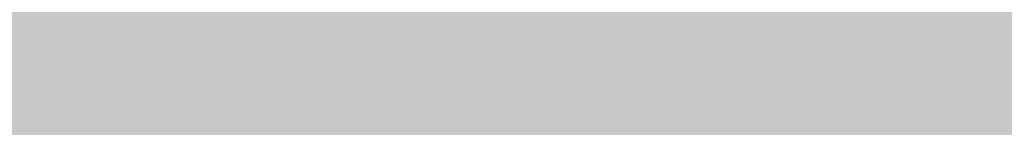
# Model space of a CAD drawing. Units: millimetres. Extents: x -22994 to 29398, y -19990 to 20176.
# Tile 71 of 135: x 226.355 to 227.437, y 83.328 to 83.446. Entities that reach past the tile are written whole.
import ezdxf
from ezdxf import colors
from ezdxf.entities.mleader import LeaderData, LeaderLine
from ezdxf.math import Vec2, Vec3

# ---------------------------------------------------------------- set-up
doc = ezdxf.new("R2010")
doc.units = ezdxf.units.MM
doc.header["$MEASUREMENT"] = 0
doc.layers.add('M-ANNO-TEXT', color=7, linetype='Continuous', lineweight=25)
doc.layers.add('M-DIMS', color=2, linetype='Continuous', lineweight=18)
doc.styles.get("Standard").update_dxf_attribs({"font": 'arial.ttf'})
doc.dimstyles.get("Standard").update_dxf_attribs({"dimtxt": 0.18, "dimasz": 10000, "dimexe": 0.18, "dimexo": 0.0625, "dimgap": 0.09, "dimtad": 0, "dimtih": 1, "dimtoh": 1, "dimdec": 0, "dimzin": 0, "dimdsep": 46, "dimtxsty": 'Standard', "dimcen": 0.09, "dimadec": 0, "dimazin": 0, "dimtfac": 1, "dimtdec": 0, "dimtofl": 0, "dimtmove": 0, "dimatfit": 3, "dimfxl": 1, "dimtolj": 1, "dimtzin": 0, "dimlwd": 30, "dimarcsym": 0})

# ---------------------------------------------------------------- blocks, each defined once
blk = doc.blocks.new('*D2')
at = {"layer": 'Defpoints', "color": 0, "transparency": 16777216}
for p in [(6.6773, 10.2713), (290.852, 10.2713), (290.852, -5.0787)]:
    blk.add_point(p, dxfattribs=at)
at = {"layer": 'M-DIMS', "color": 0, "lineweight": -2, "transparency": 16777216}
for p, q in [((6.6773, 10.2088), (6.6773, -5.2587)), ((290.852, 10.2088), (290.852, -5.2587))]:
    blk.add_line(p, q, dxfattribs=at)
at = {"layer": 'M-DIMS', "color": 0, "lineweight": 30, "transparency": 16777216}
for p, q in [((-9993.3227, -5.0787), (-19993.3227, -5.0787)), ((10290.852, -5.0787), (20290.852, -5.0787))]:
    blk.add_line(p, q, dxfattribs=at)
at = {"layer": 'M-DIMS', "color": 0, "transparency": 16777216}
for points in [[(-9993.3227, 1661.5879), (-9993.3227, -1671.7454), (6.6773, -5.0787)], [(10290.852, 1661.5879), (10290.852, -1671.7454), (290.852, -5.0787)]]:
    blk.add_solid(points, dxfattribs=at)
at = {"layer": 'M-DIMS', "color": 0, "transparency": 16777216, "insert": (148.7647, -5.0787), "char_height": 0.18, "attachment_point": 5}
blk.add_mtext('\\A1;284.2', dxfattribs=at)
blk = doc.blocks.new('*D3')
at = {"layer": 'Defpoints', "color": 0, "transparency": 16777216}
for p in [(110.2647, 204.1654), (110.2647, 176.3662), (95.8327, 127.967)]:
    blk.add_point(p, dxfattribs=at)
at = {"layer": 'M-DIMS', "color": 0, "lineweight": -2, "transparency": 16777216}
for p, q in [((95.8327, 128.0295), (95.8327, 204.3454)), ((110.2647, 176.4287), (110.2647, 204.3454))]:
    blk.add_line(p, q, dxfattribs=at)
at = {"layer": 'M-DIMS', "color": 0, "lineweight": 30, "transparency": 16777216}
for p, q in [((-9904.1673, 204.1654), (-19904.1673, 204.1654)), ((10110.2647, 204.1654), (20110.2647, 204.1654))]:
    blk.add_line(p, q, dxfattribs=at)
at = {"layer": 'M-DIMS', "color": 0, "transparency": 16777216}
for points in [[(-9904.1673, 1870.8321), (-9904.1673, -1462.5013), (95.8327, 204.1654)], [(10110.2647, 1870.8321), (10110.2647, -1462.5013), (110.2647, 204.1654)]]:
    blk.add_solid(points, dxfattribs=at)
at = {"layer": 'M-DIMS', "color": 0, "transparency": 16777216, "insert": (103.0487, 204.1654), "char_height": 0.18, "attachment_point": 5}
blk.add_mtext('\\A1;14.432', dxfattribs=at)
blk = doc.blocks.new('*D4')
at = {"layer": 'Defpoints', "color": 0, "transparency": 16777216}
for p in [(116.2647, 204.1654), (110.2647, 176.3662), (116.2647, 176.3662)]:
    blk.add_point(p, dxfattribs=at)
at = {"layer": 'M-DIMS', "color": 0, "lineweight": -2, "transparency": 16777216}
for p, q in [((110.2647, 176.4287), (110.2647, 204.3454)), ((116.2647, 176.4287), (116.2647, 204.3454))]:
    blk.add_line(p, q, dxfattribs=at)
at = {"layer": 'M-DIMS', "color": 0, "lineweight": 30, "transparency": 16777216}
for p, q in [((-9889.7353, 204.1654), (-19889.7353, 204.1654)), ((10116.2647, 204.1654), (20116.2647, 204.1654))]:
    blk.add_line(p, q, dxfattribs=at)
at = {"layer": 'M-DIMS', "color": 0, "transparency": 16777216}
for points in [[(-9889.7353, 1870.8321), (-9889.7353, -1462.5013), (110.2647, 204.1654)], [(10116.2647, 1870.8321), (10116.2647, -1462.5013), (116.2647, 204.1654)]]:
    blk.add_solid(points, dxfattribs=at)
at = {"layer": 'M-DIMS', "color": 0, "transparency": 16777216, "insert": (113.2647, 204.1654), "char_height": 0.18, "attachment_point": 5}
blk.add_mtext('\\A1;6', dxfattribs=at)
blk = doc.blocks.new('*D5')
at = {"layer": 'Defpoints', "color": 0, "transparency": 16777216}
for p in [(181.2647, 204.1654), (116.2647, 176.3662), (181.2647, 176.3662)]:
    blk.add_point(p, dxfattribs=at)
at = {"layer": 'M-DIMS', "color": 0, "lineweight": -2, "transparency": 16777216}
for p, q in [((116.2647, 176.4287), (116.2647, 204.3454)), ((181.2647, 176.4287), (181.2647, 204.3454))]:
    blk.add_line(p, q, dxfattribs=at)
at = {"layer": 'M-DIMS', "color": 0, "lineweight": 30, "transparency": 16777216}
for p, q in [((-9883.7353, 204.1654), (-19883.7353, 204.1654)), ((10181.2647, 204.1654), (20181.2647, 204.1654))]:
    blk.add_line(p, q, dxfattribs=at)
at = {"layer": 'M-DIMS', "color": 0, "transparency": 16777216}
for points in [[(-9883.7353, 1870.8321), (-9883.7353, -1462.5013), (116.2647, 204.1654)], [(10181.2647, 1870.8321), (10181.2647, -1462.5013), (181.2647, 204.1654)]]:
    blk.add_solid(points, dxfattribs=at)
at = {"layer": 'M-DIMS', "color": 0, "transparency": 16777216, "insert": (148.7647, 204.1654), "char_height": 0.18, "attachment_point": 5}
blk.add_mtext('\\A1;65', dxfattribs=at)
blk = doc.blocks.new('*D6')
at = {"layer": 'Defpoints', "color": 0, "transparency": 16777216}
for p in [(187.2647, 204.1654), (181.2647, 176.3662), (187.2647, 176.3662)]:
    blk.add_point(p, dxfattribs=at)
at = {"layer": 'M-DIMS', "color": 0, "lineweight": -2, "transparency": 16777216}
for p, q in [((181.2647, 176.4287), (181.2647, 204.3454)), ((187.2647, 176.4287), (187.2647, 204.3454))]:
    blk.add_line(p, q, dxfattribs=at)
at = {"layer": 'M-DIMS', "color": 0, "lineweight": 30, "transparency": 16777216}
for p, q in [((-9818.7353, 204.1654), (-19818.7353, 204.1654)), ((10187.2647, 204.1654), (20187.2647, 204.1654))]:
    blk.add_line(p, q, dxfattribs=at)
at = {"layer": 'M-DIMS', "color": 0, "transparency": 16777216}
for points in [[(-9818.7353, 1870.8321), (-9818.7353, -1462.5013), (181.2647, 204.1654)], [(10187.2647, 1870.8321), (10187.2647, -1462.5013), (187.2647, 204.1654)]]:
    blk.add_solid(points, dxfattribs=at)
at = {"layer": 'M-DIMS', "color": 0, "transparency": 16777216, "insert": (184.2647, 204.1654), "char_height": 0.18, "attachment_point": 5}
blk.add_mtext('\\A1;6', dxfattribs=at)
blk = doc.blocks.new('*D7')
at = {"layer": 'Defpoints', "color": 0, "transparency": 16777216}
for p in [(201.6967, 204.1654), (187.2647, 176.3662), (201.6967, 127.967)]:
    blk.add_point(p, dxfattribs=at)
at = {"layer": 'M-DIMS', "color": 0, "lineweight": -2, "transparency": 16777216}
for p, q in [((187.2647, 176.4287), (187.2647, 204.3454)), ((201.6967, 128.0295), (201.6967, 204.3454))]:
    blk.add_line(p, q, dxfattribs=at)
at = {"layer": 'M-DIMS', "color": 0, "lineweight": 30, "transparency": 16777216}
for p, q in [((-9812.7353, 204.1654), (-19812.7353, 204.1654)), ((10201.6967, 204.1654), (20201.6967, 204.1654))]:
    blk.add_line(p, q, dxfattribs=at)
at = {"layer": 'M-DIMS', "color": 0, "transparency": 16777216}
for points in [[(-9812.7353, 1870.8321), (-9812.7353, -1462.5013), (187.2647, 204.1654)], [(10201.6967, 1870.8321), (10201.6967, -1462.5013), (201.6967, 204.1654)]]:
    blk.add_solid(points, dxfattribs=at)
at = {"layer": 'M-DIMS', "color": 0, "transparency": 16777216, "insert": (194.4807, 204.1654), "char_height": 0.18, "attachment_point": 5}
blk.add_mtext('\\A1;14.432', dxfattribs=at)
blk = doc.blocks.new('*D8')
at = {"layer": 'Defpoints', "color": 0, "transparency": 16777216}
for p in [(227.6485, 204.1654), (227.6485, 146.7296), (201.6967, 127.967)]:
    blk.add_point(p, dxfattribs=at)
at = {"layer": 'M-DIMS', "color": 0, "lineweight": -2, "transparency": 16777216}
for p, q in [((201.6967, 128.0295), (201.6967, 204.3454)), ((227.6485, 146.7921), (227.6485, 204.3454))]:
    blk.add_line(p, q, dxfattribs=at)
at = {"layer": 'M-DIMS', "color": 0, "lineweight": 30, "transparency": 16777216}
for p, q in [((-9798.3033, 204.1654), (-19798.3033, 204.1654)), ((10227.6485, 204.1654), (20227.6485, 204.1654))]:
    blk.add_line(p, q, dxfattribs=at)
at = {"layer": 'M-DIMS', "color": 0, "transparency": 16777216}
for points in [[(-9798.3033, 1870.8321), (-9798.3033, -1462.5013), (201.6967, 204.1654)], [(10227.6485, 1870.8321), (10227.6485, -1462.5013), (227.6485, 204.1654)]]:
    blk.add_solid(points, dxfattribs=at)
at = {"layer": 'M-DIMS', "color": 0, "transparency": 16777216, "insert": (214.6726, 204.1654), "char_height": 0.18, "attachment_point": 5}
blk.add_mtext('\\A1;25.95', dxfattribs=at)
blk = doc.blocks.new('*D9')
at = {"layer": 'Defpoints', "color": 0, "transparency": 16777216}
for p in [(187.2647, 176.3662), (306.202, 176.3662), (290.852, 10.2713)]:
    blk.add_point(p, dxfattribs=at)
at = {"layer": 'M-DIMS', "color": 0, "lineweight": 30, "transparency": 16777216}
for p, q in [((306.202, 10176.3662), (306.202, 20176.3662)), ((306.202, -9989.7287), (306.202, -19989.7287))]:
    blk.add_line(p, q, dxfattribs=at)
at = {"layer": 'M-DIMS', "color": 0, "lineweight": -2, "transparency": 16777216}
for p, q in [((187.3272, 176.3662), (306.382, 176.3662)), ((290.9145, 10.2713), (306.382, 10.2713))]:
    blk.add_line(p, q, dxfattribs=at)
at = {"layer": 'M-DIMS', "color": 0, "transparency": 16777216}
for points in [[(-1360.4646, 10176.3662), (1972.8687, 10176.3662), (306.202, 176.3662)], [(-1360.4646, -9989.7287), (1972.8687, -9989.7287), (306.202, 10.2713)]]:
    blk.add_solid(points, dxfattribs=at)
at = {"layer": 'M-DIMS', "color": 0, "transparency": 16777216, "insert": (306.202, 93.3187), "char_height": 0.18, "attachment_point": 5}
blk.add_mtext('\\A1;166.1', dxfattribs=at)
blk = doc.blocks.new('*D10')
at = {"layer": 'Defpoints', "color": 0, "transparency": 16777216}
for p in [(125.6498, 136.0713), (133.3459, 136.0713), (133.3459, -5.0787)]:
    blk.add_point(p, dxfattribs=at)
at = {"layer": 'M-DIMS', "color": 0, "lineweight": -2, "transparency": 16777216}
for p, q in [((125.6498, 136.0088), (125.6498, -5.2587)), ((133.3459, 136.0088), (133.3459, -5.2587))]:
    blk.add_line(p, q, dxfattribs=at)
at = {"layer": 'M-DIMS', "color": 0, "lineweight": 30, "transparency": 16777216}
for p, q in [((-9874.3502, -5.0787), (-19874.3502, -5.0787)), ((10133.3459, -5.0787), (20133.3459, -5.0787))]:
    blk.add_line(p, q, dxfattribs=at)
at = {"layer": 'M-DIMS', "color": 0, "transparency": 16777216}
for points in [[(-9874.3502, 1661.5879), (-9874.3502, -1671.7454), (125.6498, -5.0787)], [(10133.3459, 1661.5879), (10133.3459, -1671.7454), (133.3459, -5.0787)]]:
    blk.add_solid(points, dxfattribs=at)
at = {"layer": 'M-DIMS', "color": 0, "transparency": 16777216, "insert": (129.4978, -5.0787), "char_height": 0.18, "attachment_point": 5}
blk.add_mtext('\\A1;7.696', dxfattribs=at)
blk = doc.blocks.new('*D11')
at = {"layer": 'Defpoints', "color": 0, "transparency": 16777216}
for p in [(133.3459, 136.0713), (135.6498, 136.0713), (135.6498, -5.0787)]:
    blk.add_point(p, dxfattribs=at)
at = {"layer": 'M-DIMS', "color": 0, "lineweight": -2, "transparency": 16777216}
for p, q in [((133.3459, 136.0088), (133.3459, -5.2587)), ((135.6498, 136.0088), (135.6498, -5.2587))]:
    blk.add_line(p, q, dxfattribs=at)
at = {"layer": 'M-DIMS', "color": 0, "lineweight": 30, "transparency": 16777216}
for p, q in [((-9866.6541, -5.0787), (-19866.6541, -5.0787)), ((10135.6498, -5.0787), (20135.6498, -5.0787))]:
    blk.add_line(p, q, dxfattribs=at)
at = {"layer": 'M-DIMS', "color": 0, "transparency": 16777216}
for points in [[(-9866.6541, 1661.5879), (-9866.6541, -1671.7454), (133.3459, -5.0787)], [(10135.6498, 1661.5879), (10135.6498, -1671.7454), (135.6498, -5.0787)]]:
    blk.add_solid(points, dxfattribs=at)
at = {"layer": 'M-DIMS', "color": 0, "transparency": 16777216, "insert": (134.4978, -5.0787), "char_height": 0.18, "attachment_point": 5}
blk.add_mtext('\\A1;2.304', dxfattribs=at)
blk = doc.blocks.new('*D12')
at = {"layer": 'Defpoints', "color": 0, "transparency": 16777216}
for p in [(135.6498, 136.0713), (145.6498, 136.0713), (145.6498, -5.0787)]:
    blk.add_point(p, dxfattribs=at)
at = {"layer": 'M-DIMS', "color": 0, "lineweight": -2, "transparency": 16777216}
for p, q in [((135.6498, 136.0088), (135.6498, -5.2587)), ((145.6498, 136.0088), (145.6498, -5.2587))]:
    blk.add_line(p, q, dxfattribs=at)
at = {"layer": 'M-DIMS', "color": 0, "lineweight": 30, "transparency": 16777216}
for p, q in [((-9864.3502, -5.0787), (-19864.3502, -5.0787)), ((10145.6498, -5.0787), (20145.6498, -5.0787))]:
    blk.add_line(p, q, dxfattribs=at)
at = {"layer": 'M-DIMS', "color": 0, "transparency": 16777216}
for points in [[(-9864.3502, 1661.5879), (-9864.3502, -1671.7454), (135.6498, -5.0787)], [(10145.6498, 1661.5879), (10145.6498, -1671.7454), (145.6498, -5.0787)]]:
    blk.add_solid(points, dxfattribs=at)
at = {"layer": 'M-DIMS', "color": 0, "transparency": 16777216, "insert": (140.6498, -5.0787), "char_height": 0.18, "attachment_point": 5}
blk.add_mtext('\\A1;10', dxfattribs=at)
blk = doc.blocks.new('*D13')
at = {"layer": 'Defpoints', "color": 0, "transparency": 16777216}
for p in [(145.6498, 136.0713), (155.6498, 136.0713), (155.6498, -5.0787)]:
    blk.add_point(p, dxfattribs=at)
at = {"layer": 'M-DIMS', "color": 0, "lineweight": -2, "transparency": 16777216}
for p, q in [((145.6498, 136.0088), (145.6498, -5.2587)), ((155.6498, 136.0088), (155.6498, -5.2587))]:
    blk.add_line(p, q, dxfattribs=at)
at = {"layer": 'M-DIMS', "color": 0, "lineweight": 30, "transparency": 16777216}
for p, q in [((-9854.3502, -5.0787), (-19854.3502, -5.0787)), ((10155.6498, -5.0787), (20155.6498, -5.0787))]:
    blk.add_line(p, q, dxfattribs=at)
at = {"layer": 'M-DIMS', "color": 0, "transparency": 16777216}
for points in [[(-9854.3502, 1661.5879), (-9854.3502, -1671.7454), (145.6498, -5.0787)], [(10155.6498, 1661.5879), (10155.6498, -1671.7454), (155.6498, -5.0787)]]:
    blk.add_solid(points, dxfattribs=at)
at = {"layer": 'M-DIMS', "color": 0, "transparency": 16777216, "insert": (150.6498, -5.0787), "char_height": 0.18, "attachment_point": 5}
blk.add_mtext('\\A1;10', dxfattribs=at)
blk = doc.blocks.new('*D14')
at = {"layer": 'Defpoints', "color": 0, "transparency": 16777216}
for p in [(155.6498, 136.0713), (165.6498, 136.0713), (165.6498, -5.0787)]:
    blk.add_point(p, dxfattribs=at)
at = {"layer": 'M-DIMS', "color": 0, "lineweight": -2, "transparency": 16777216}
for p, q in [((155.6498, 136.0088), (155.6498, -5.2587)), ((165.6498, 136.0088), (165.6498, -5.2587))]:
    blk.add_line(p, q, dxfattribs=at)
at = {"layer": 'M-DIMS', "color": 0, "lineweight": 30, "transparency": 16777216}
for p, q in [((-9844.3502, -5.0787), (-19844.3502, -5.0787)), ((10165.6498, -5.0787), (20165.6498, -5.0787))]:
    blk.add_line(p, q, dxfattribs=at)
at = {"layer": 'M-DIMS', "color": 0, "transparency": 16777216}
for points in [[(-9844.3502, 1661.5879), (-9844.3502, -1671.7454), (155.6498, -5.0787)], [(10165.6498, 1661.5879), (10165.6498, -1671.7454), (165.6498, -5.0787)]]:
    blk.add_solid(points, dxfattribs=at)
at = {"layer": 'M-DIMS', "color": 0, "transparency": 16777216, "insert": (160.6498, -5.0787), "char_height": 0.18, "attachment_point": 5}
blk.add_mtext('\\A1;10', dxfattribs=at)
blk = doc.blocks.new('*D15')
at = {"layer": 'Defpoints', "color": 0, "transparency": 16777216}
for p in [(173.3459, 154.788), (173.3459, 136.0713), (306.202, 136.0713)]:
    blk.add_point(p, dxfattribs=at)
at = {"layer": 'M-DIMS', "color": 0, "lineweight": 30, "transparency": 16777216}
for p, q in [((306.202, 10154.788), (306.202, 20154.788)), ((306.202, -9863.9287), (306.202, -19863.9287))]:
    blk.add_line(p, q, dxfattribs=at)
at = {"layer": 'M-DIMS', "color": 0, "lineweight": -2, "transparency": 16777216}
for p, q in [((173.4084, 154.788), (306.382, 154.788)), ((173.4084, 136.0713), (306.382, 136.0713))]:
    blk.add_line(p, q, dxfattribs=at)
at = {"layer": 'M-DIMS', "color": 0, "transparency": 16777216}
for points in [[(-1360.4646, 10154.788), (1972.8687, 10154.788), (306.202, 154.788)], [(-1360.4646, -9863.9287), (1972.8687, -9863.9287), (306.202, 136.0713)]]:
    blk.add_solid(points, dxfattribs=at)
at = {"layer": 'M-DIMS', "color": 0, "transparency": 16777216, "insert": (306.202, 145.4297), "char_height": 0.18, "attachment_point": 5}
blk.add_mtext('\\A1;18.717', dxfattribs=at)
blk = doc.blocks.new('*D16')
at = {"layer": 'Defpoints', "color": 0, "transparency": 16777216}
for p in [(120.1702, 204.1654), (110.4658, 48.0349), (120.1702, 48.0349)]:
    blk.add_point(p, dxfattribs=at)
at = {"layer": 'M-DIMS', "color": 0, "lineweight": -2, "transparency": 16777216}
for p, q in [((110.4658, 48.0974), (110.4658, 204.3454)), ((120.1702, 48.0974), (120.1702, 204.3454))]:
    blk.add_line(p, q, dxfattribs=at)
at = {"layer": 'M-DIMS', "color": 0, "lineweight": 30, "transparency": 16777216}
for p, q in [((-9889.5342, 204.1654), (-19889.5342, 204.1654)), ((10120.1702, 204.1654), (20120.1702, 204.1654))]:
    blk.add_line(p, q, dxfattribs=at)
at = {"layer": 'M-DIMS', "color": 0, "transparency": 16777216}
for points in [[(-9889.5342, 1870.8321), (-9889.5342, -1462.5013), (110.4658, 204.1654)], [(10120.1702, 1870.8321), (10120.1702, -1462.5013), (120.1702, 204.1654)]]:
    blk.add_solid(points, dxfattribs=at)
at = {"layer": 'M-DIMS', "color": 0, "transparency": 16777216, "insert": (115.318, 204.1654), "char_height": 0.18, "attachment_point": 5}
blk.add_mtext('\\A1;9.704', dxfattribs=at)
blk = doc.blocks.new('*D17')
at = {"layer": 'Defpoints', "color": 0, "transparency": 16777216}
for p in [(126.1702, 204.1654), (120.1702, 48.0349), (126.1702, 48.0349)]:
    blk.add_point(p, dxfattribs=at)
at = {"layer": 'M-DIMS', "color": 0, "lineweight": -2, "transparency": 16777216}
for p, q in [((120.1702, 48.0974), (120.1702, 204.3454)), ((126.1702, 48.0974), (126.1702, 204.3454))]:
    blk.add_line(p, q, dxfattribs=at)
at = {"layer": 'M-DIMS', "color": 0, "lineweight": 30, "transparency": 16777216}
for p, q in [((-9879.8298, 204.1654), (-19879.8298, 204.1654)), ((10126.1702, 204.1654), (20126.1702, 204.1654))]:
    blk.add_line(p, q, dxfattribs=at)
at = {"layer": 'M-DIMS', "color": 0, "transparency": 16777216}
for points in [[(-9879.8298, 1870.8321), (-9879.8298, -1462.5013), (120.1702, 204.1654)], [(10126.1702, 1870.8321), (10126.1702, -1462.5013), (126.1702, 204.1654)]]:
    blk.add_solid(points, dxfattribs=at)
at = {"layer": 'M-DIMS', "color": 0, "transparency": 16777216, "insert": (123.1702, 204.1654), "char_height": 0.18, "attachment_point": 5}
blk.add_mtext('\\A1;6', dxfattribs=at)
blk = doc.blocks.new('*D18')
at = {"layer": 'Defpoints', "color": 0, "transparency": 16777216}
for p in [(132.1702, 204.1654), (126.1702, 48.0349), (132.1702, 48.0349)]:
    blk.add_point(p, dxfattribs=at)
at = {"layer": 'M-DIMS', "color": 0, "lineweight": -2, "transparency": 16777216}
for p, q in [((126.1702, 48.0974), (126.1702, 204.3454)), ((132.1702, 48.0974), (132.1702, 204.3454))]:
    blk.add_line(p, q, dxfattribs=at)
at = {"layer": 'M-DIMS', "color": 0, "lineweight": 30, "transparency": 16777216}
for p, q in [((-9873.8298, 204.1654), (-19873.8298, 204.1654)), ((10132.1702, 204.1654), (20132.1702, 204.1654))]:
    blk.add_line(p, q, dxfattribs=at)
at = {"layer": 'M-DIMS', "color": 0, "transparency": 16777216}
for points in [[(-9873.8298, 1870.8321), (-9873.8298, -1462.5013), (126.1702, 204.1654)], [(10132.1702, 1870.8321), (10132.1702, -1462.5013), (132.1702, 204.1654)]]:
    blk.add_solid(points, dxfattribs=at)
at = {"layer": 'M-DIMS', "color": 0, "transparency": 16777216, "insert": (129.1702, 204.1654), "char_height": 0.18, "attachment_point": 5}
blk.add_mtext('\\A1;6', dxfattribs=at)
blk = doc.blocks.new('*D19')
at = {"layer": 'Defpoints', "color": 0, "transparency": 16777216}
for p in [(138.1702, 204.1654), (132.1702, 48.0349), (138.1702, 48.0349)]:
    blk.add_point(p, dxfattribs=at)
at = {"layer": 'M-DIMS', "color": 0, "lineweight": -2, "transparency": 16777216}
for p, q in [((132.1702, 48.0974), (132.1702, 204.3454)), ((138.1702, 48.0974), (138.1702, 204.3454))]:
    blk.add_line(p, q, dxfattribs=at)
at = {"layer": 'M-DIMS', "color": 0, "lineweight": 30, "transparency": 16777216}
for p, q in [((-9867.8298, 204.1654), (-19867.8298, 204.1654)), ((10138.1702, 204.1654), (20138.1702, 204.1654))]:
    blk.add_line(p, q, dxfattribs=at)
at = {"layer": 'M-DIMS', "color": 0, "transparency": 16777216}
for points in [[(-9867.8298, 1870.8321), (-9867.8298, -1462.5013), (132.1702, 204.1654)], [(10138.1702, 1870.8321), (10138.1702, -1462.5013), (138.1702, 204.1654)]]:
    blk.add_solid(points, dxfattribs=at)
at = {"layer": 'M-DIMS', "color": 0, "transparency": 16777216, "insert": (135.1702, 204.1654), "char_height": 0.18, "attachment_point": 5}
blk.add_mtext('\\A1;6', dxfattribs=at)
blk = doc.blocks.new('*D20')
at = {"layer": 'Defpoints', "color": 0, "transparency": 16777216}
for p in [(144.1702, 204.1654), (138.1702, 48.0349), (144.1702, 48.0349)]:
    blk.add_point(p, dxfattribs=at)
at = {"layer": 'M-DIMS', "color": 0, "lineweight": -2, "transparency": 16777216}
for p, q in [((138.1702, 48.0974), (138.1702, 204.3454)), ((144.1702, 48.0974), (144.1702, 204.3454))]:
    blk.add_line(p, q, dxfattribs=at)
at = {"layer": 'M-DIMS', "color": 0, "lineweight": 30, "transparency": 16777216}
for p, q in [((-9861.8298, 204.1654), (-19861.8298, 204.1654)), ((10144.1702, 204.1654), (20144.1702, 204.1654))]:
    blk.add_line(p, q, dxfattribs=at)
at = {"layer": 'M-DIMS', "color": 0, "transparency": 16777216}
for points in [[(-9861.8298, 1870.8321), (-9861.8298, -1462.5013), (138.1702, 204.1654)], [(10144.1702, 1870.8321), (10144.1702, -1462.5013), (144.1702, 204.1654)]]:
    blk.add_solid(points, dxfattribs=at)
at = {"layer": 'M-DIMS', "color": 0, "transparency": 16777216, "insert": (141.1702, 204.1654), "char_height": 0.18, "attachment_point": 5}
blk.add_mtext('\\A1;6', dxfattribs=at)
blk = doc.blocks.new('*D21')
at = {"layer": 'Defpoints', "color": 0, "transparency": 16777216}
for p in [(149.1157, 204.1654), (144.1702, 48.0349), (149.1157, 48.0349)]:
    blk.add_point(p, dxfattribs=at)
at = {"layer": 'M-DIMS', "color": 0, "lineweight": -2, "transparency": 16777216}
for p, q in [((144.1702, 48.0974), (144.1702, 204.3454)), ((149.1157, 48.0974), (149.1157, 204.3454))]:
    blk.add_line(p, q, dxfattribs=at)
at = {"layer": 'M-DIMS', "color": 0, "lineweight": 30, "transparency": 16777216}
for p, q in [((-9855.8298, 204.1654), (-19855.8298, 204.1654)), ((10149.1157, 204.1654), (20149.1157, 204.1654))]:
    blk.add_line(p, q, dxfattribs=at)
at = {"layer": 'M-DIMS', "color": 0, "transparency": 16777216}
for points in [[(-9855.8298, 1870.8321), (-9855.8298, -1462.5013), (144.1702, 204.1654)], [(10149.1157, 1870.8321), (10149.1157, -1462.5013), (149.1157, 204.1654)]]:
    blk.add_solid(points, dxfattribs=at)
at = {"layer": 'M-DIMS', "color": 0, "transparency": 16777216, "insert": (146.6429, 204.1654), "char_height": 0.18, "attachment_point": 5}
blk.add_mtext('\\A1;4.945', dxfattribs=at)
blk = doc.blocks.new('*D22')
at = {"layer": 'Defpoints', "color": 0, "transparency": 16777216}
for p in [(149.1157, 30.9895), (155.1157, 30.9895), (155.1157, -5.0787)]:
    blk.add_point(p, dxfattribs=at)
at = {"layer": 'M-DIMS', "color": 0, "lineweight": -2, "transparency": 16777216}
for p, q in [((149.1157, 30.927), (149.1157, -5.2587)), ((155.1157, 30.927), (155.1157, -5.2587))]:
    blk.add_line(p, q, dxfattribs=at)
at = {"layer": 'M-DIMS', "color": 0, "lineweight": 30, "transparency": 16777216}
for p, q in [((-9850.8843, -5.0787), (-19850.8843, -5.0787)), ((10155.1157, -5.0787), (20155.1157, -5.0787))]:
    blk.add_line(p, q, dxfattribs=at)
at = {"layer": 'M-DIMS', "color": 0, "transparency": 16777216}
for points in [[(-9850.8843, 1661.5879), (-9850.8843, -1671.7454), (149.1157, -5.0787)], [(10155.1157, 1661.5879), (10155.1157, -1671.7454), (155.1157, -5.0787)]]:
    blk.add_solid(points, dxfattribs=at)
at = {"layer": 'M-DIMS', "color": 0, "transparency": 16777216, "insert": (152.1157, -5.0787), "char_height": 0.18, "attachment_point": 5}
blk.add_mtext('\\A1;6', dxfattribs=at)
blk = doc.blocks.new('*D23')
at = {"layer": 'Defpoints', "color": 0, "transparency": 16777216}
for p in [(155.1157, 30.9895), (161.1157, 30.9895), (161.1157, -5.0787)]:
    blk.add_point(p, dxfattribs=at)
at = {"layer": 'M-DIMS', "color": 0, "lineweight": -2, "transparency": 16777216}
for p, q in [((155.1157, 30.927), (155.1157, -5.2587)), ((161.1157, 30.927), (161.1157, -5.2587))]:
    blk.add_line(p, q, dxfattribs=at)
at = {"layer": 'M-DIMS', "color": 0, "lineweight": 30, "transparency": 16777216}
for p, q in [((-9844.8843, -5.0787), (-19844.8843, -5.0787)), ((10161.1157, -5.0787), (20161.1157, -5.0787))]:
    blk.add_line(p, q, dxfattribs=at)
at = {"layer": 'M-DIMS', "color": 0, "transparency": 16777216}
for points in [[(-9844.8843, 1661.5879), (-9844.8843, -1671.7454), (155.1157, -5.0787)], [(10161.1157, 1661.5879), (10161.1157, -1671.7454), (161.1157, -5.0787)]]:
    blk.add_solid(points, dxfattribs=at)
at = {"layer": 'M-DIMS', "color": 0, "transparency": 16777216, "insert": (158.1157, -5.0787), "char_height": 0.18, "attachment_point": 5}
blk.add_mtext('\\A1;6', dxfattribs=at)
blk = doc.blocks.new('*D24')
at = {"layer": 'Defpoints', "color": 0, "transparency": 16777216}
for p in [(161.1157, 30.9895), (166.4387, 30.9895), (166.4387, -5.0787)]:
    blk.add_point(p, dxfattribs=at)
at = {"layer": 'M-DIMS', "color": 0, "lineweight": -2, "transparency": 16777216}
for p, q in [((161.1157, 30.927), (161.1157, -5.2587)), ((166.4387, 30.927), (166.4387, -5.2587))]:
    blk.add_line(p, q, dxfattribs=at)
at = {"layer": 'M-DIMS', "color": 0, "lineweight": 30, "transparency": 16777216}
for p, q in [((-9838.8843, -5.0787), (-19838.8843, -5.0787)), ((10166.4387, -5.0787), (20166.4387, -5.0787))]:
    blk.add_line(p, q, dxfattribs=at)
at = {"layer": 'M-DIMS', "color": 0, "transparency": 16777216}
for points in [[(-9838.8843, 1661.5879), (-9838.8843, -1671.7454), (161.1157, -5.0787)], [(10166.4387, 1661.5879), (10166.4387, -1671.7454), (166.4387, -5.0787)]]:
    blk.add_solid(points, dxfattribs=at)
at = {"layer": 'M-DIMS', "color": 0, "transparency": 16777216, "insert": (163.7772, -5.0787), "char_height": 0.18, "attachment_point": 5}
blk.add_mtext('\\A1;5.323', dxfattribs=at)
blk = doc.blocks.new('*D25')
at = {"layer": 'Defpoints', "color": 0, "transparency": 16777216}
for p in [(166.4387, 30.9895), (172.4387, 30.9895), (172.4387, -5.0787)]:
    blk.add_point(p, dxfattribs=at)
at = {"layer": 'M-DIMS', "color": 0, "lineweight": -2, "transparency": 16777216}
for p, q in [((166.4387, 30.927), (166.4387, -5.2587)), ((172.4387, 30.927), (172.4387, -5.2587))]:
    blk.add_line(p, q, dxfattribs=at)
at = {"layer": 'M-DIMS', "color": 0, "lineweight": 30, "transparency": 16777216}
for p, q in [((-9833.5613, -5.0787), (-19833.5613, -5.0787)), ((10172.4387, -5.0787), (20172.4387, -5.0787))]:
    blk.add_line(p, q, dxfattribs=at)
at = {"layer": 'M-DIMS', "color": 0, "transparency": 16777216}
for points in [[(-9833.5613, 1661.5879), (-9833.5613, -1671.7454), (166.4387, -5.0787)], [(10172.4387, 1661.5879), (10172.4387, -1671.7454), (172.4387, -5.0787)]]:
    blk.add_solid(points, dxfattribs=at)
at = {"layer": 'M-DIMS', "color": 0, "transparency": 16777216, "insert": (169.4387, -5.0787), "char_height": 0.18, "attachment_point": 5}
blk.add_mtext('\\A1;6', dxfattribs=at)
blk = doc.blocks.new('*D26')
at = {"layer": 'Defpoints', "color": 0, "transparency": 16777216}
for p in [(172.4387, 30.9895), (178.4387, 30.9895), (178.4387, -5.0787)]:
    blk.add_point(p, dxfattribs=at)
at = {"layer": 'M-DIMS', "color": 0, "lineweight": -2, "transparency": 16777216}
for p, q in [((172.4387, 30.927), (172.4387, -5.2587)), ((178.4387, 30.927), (178.4387, -5.2587))]:
    blk.add_line(p, q, dxfattribs=at)
at = {"layer": 'M-DIMS', "color": 0, "lineweight": 30, "transparency": 16777216}
for p, q in [((-9827.5613, -5.0787), (-19827.5613, -5.0787)), ((10178.4387, -5.0787), (20178.4387, -5.0787))]:
    blk.add_line(p, q, dxfattribs=at)
at = {"layer": 'M-DIMS', "color": 0, "transparency": 16777216}
for points in [[(-9827.5613, 1661.5879), (-9827.5613, -1671.7454), (172.4387, -5.0787)], [(10178.4387, 1661.5879), (10178.4387, -1671.7454), (178.4387, -5.0787)]]:
    blk.add_solid(points, dxfattribs=at)
at = {"layer": 'M-DIMS', "color": 0, "transparency": 16777216, "insert": (175.4387, -5.0787), "char_height": 0.18, "attachment_point": 5}
blk.add_mtext('\\A1;6', dxfattribs=at)
blk = doc.blocks.new('*D27')
at = {"layer": 'Defpoints', "color": 0, "transparency": 16777216}
for p in [(178.4387, 30.9895), (188.1175, 30.9895), (188.1175, -5.0787)]:
    blk.add_point(p, dxfattribs=at)
at = {"layer": 'M-DIMS', "color": 0, "lineweight": -2, "transparency": 16777216}
for p, q in [((178.4387, 30.927), (178.4387, -5.2587)), ((188.1175, 30.927), (188.1175, -5.2587))]:
    blk.add_line(p, q, dxfattribs=at)
at = {"layer": 'M-DIMS', "color": 0, "lineweight": 30, "transparency": 16777216}
for p, q in [((-9821.5613, -5.0787), (-19821.5613, -5.0787)), ((10188.1175, -5.0787), (20188.1175, -5.0787))]:
    blk.add_line(p, q, dxfattribs=at)
at = {"layer": 'M-DIMS', "color": 0, "transparency": 16777216}
for points in [[(-9821.5613, 1661.5879), (-9821.5613, -1671.7454), (178.4387, -5.0787)], [(10188.1175, 1661.5879), (10188.1175, -1671.7454), (188.1175, -5.0787)]]:
    blk.add_solid(points, dxfattribs=at)
at = {"layer": 'M-DIMS', "color": 0, "transparency": 16777216, "insert": (183.2781, -5.0787), "char_height": 0.18, "attachment_point": 5}
blk.add_mtext('\\A1;9.679', dxfattribs=at)
blk = doc.blocks.new('*D28')
at = {"layer": 'Defpoints', "color": 0, "transparency": 16777216}
for p in [(188.1175, 48.0349), (306.202, 48.0349), (188.1175, 30.9895)]:
    blk.add_point(p, dxfattribs=at)
at = {"layer": 'M-DIMS', "color": 0, "lineweight": 30, "transparency": 16777216}
for p, q in [((306.202, 10048.0349), (306.202, 20048.0349)), ((306.202, -9969.0105), (306.202, -19969.0105))]:
    blk.add_line(p, q, dxfattribs=at)
at = {"layer": 'M-DIMS', "color": 0, "lineweight": -2, "transparency": 16777216}
for p, q in [((188.18, 48.0349), (306.382, 48.0349)), ((188.18, 30.9895), (306.382, 30.9895))]:
    blk.add_line(p, q, dxfattribs=at)
at = {"layer": 'M-DIMS', "color": 0, "transparency": 16777216}
for points in [[(-1360.4646, 10048.0349), (1972.8687, 10048.0349), (306.202, 48.0349)], [(-1360.4646, -9969.0105), (1972.8687, -9969.0105), (306.202, 30.9895)]]:
    blk.add_solid(points, dxfattribs=at)
at = {"layer": 'M-DIMS', "color": 0, "transparency": 16777216, "insert": (306.202, 39.5122), "char_height": 0.18, "attachment_point": 5}
blk.add_mtext('\\A1;17.045', dxfattribs=at)
blk = doc.blocks.new('*D29')
at = {"layer": 'Defpoints', "color": 0, "transparency": 16777216}
for p in [(36.8006, 80.045), (64.0296, 80.045)]:
    blk.add_point(p, dxfattribs=at)
at = {"layer": 'M-DIMS', "color": 0, "lineweight": -2, "transparency": 16777216}
for p, q in [((50.4151, 79.955), (50.4151, 80.135)), ((50.3251, 80.045), (50.5051, 80.045))]:
    blk.add_line(p, q, dxfattribs=at)
at = {"layer": 'M-DIMS', "color": 0, "lineweight": 30, "transparency": 16777216}
blk.add_line((20064.0296, 80.0303), (10064.0296, 80.0377), dxfattribs=at)
at = {"layer": 'M-DIMS', "color": 0, "transparency": 16777216}
blk.add_solid([(10064.0309, 1746.7043), (10064.0284, -1586.629), (64.0296, 80.045)], dxfattribs=at)
at = {"layer": 'M-DIMS', "color": 0, "transparency": 16777216, "insert": (20064.5213, 80.0303), "char_height": 0.18, "attachment_point": 5}
blk.add_mtext('\\A1;∅27.23', dxfattribs=at)
blk = doc.blocks.new('*D30')
at = {"layer": 'Defpoints', "color": 0, "transparency": 16777216}
for p in [(216.3148, 146.7291), (238.9821, 146.73)]:
    blk.add_point(p, dxfattribs=at)
at = {"layer": 'M-DIMS', "color": 0, "lineweight": 30, "transparency": 16777216}
blk.add_line((20238.9821, 147.4959), (10238.9821, 147.1129), dxfattribs=at)
at = {"layer": 'M-DIMS', "color": 0, "lineweight": -2, "transparency": 16777216}
for p, q in [((227.6485, 146.6396), (227.6485, 146.8196)), ((227.5585, 146.7296), (227.7385, 146.7296))]:
    blk.add_line(p, q, dxfattribs=at)
at = {"layer": 'M-DIMS', "color": 0, "transparency": 16777216}
blk.add_solid([(10238.9183, 1813.7796), (10239.0459, -1519.5537), (238.9821, 146.73)], dxfattribs=at)
at = {"layer": 'M-DIMS', "color": 0, "transparency": 16777216, "insert": (20239.5436, 147.4959), "char_height": 0.18, "attachment_point": 5}
blk.add_mtext('\\A1;∅22.667', dxfattribs=at)
blk = doc.blocks.new('*D31')
at = {"layer": 'Defpoints', "color": 0, "transparency": 16777216}
for p in [(223.1641, 146.7291), (232.1328, 146.73)]:
    blk.add_point(p, dxfattribs=at)
at = {"layer": 'M-DIMS', "color": 0, "lineweight": 30, "transparency": 16777216}
blk.add_line((20232.1327, 148.6656), (10232.1328, 147.6978), dxfattribs=at)
at = {"layer": 'M-DIMS', "color": 0, "lineweight": -2, "transparency": 16777216}
for p, q in [((227.6485, 146.6396), (227.6485, 146.8196)), ((227.5585, 146.7296), (227.7385, 146.7296))]:
    blk.add_line(p, q, dxfattribs=at)
at = {"layer": 'M-DIMS', "color": 0, "transparency": 16777216}
blk.add_solid([(10231.9715, 1814.3645), (10232.2941, -1518.9688), (232.1328, 146.73)], dxfattribs=at)
at = {"layer": 'M-DIMS', "color": 0, "transparency": 16777216, "insert": (20232.6245, 148.6656), "char_height": 0.18, "attachment_point": 5}
blk.add_mtext('\\A1;∅8.969', dxfattribs=at)
blk = doc.blocks.new('*D36')
at = {"layer": 'Defpoints', "color": 0, "transparency": 16777216}
for p in [(46.39, 31.3035), (46.3875, 26.5934)]:
    blk.add_point(p, dxfattribs=at)
at = {"layer": 'M-DIMS', "color": 0, "lineweight": 30, "transparency": 16777216}
for p, q in [((57.1499, 20031.3006), (51.77, 10031.302)), ((10057.1499, 20031.3006), (57.1499, 20031.3006))]:
    blk.add_line(p, q, dxfattribs=at)
at = {"layer": 'M-DIMS', "color": 0, "lineweight": -2, "transparency": 16777216}
for p, q in [((46.3887, 28.8585), (46.3887, 29.0385)), ((46.2987, 28.9485), (46.4787, 28.9485))]:
    blk.add_line(p, q, dxfattribs=at)
at = {"layer": 'M-DIMS', "color": 0, "transparency": 16777216}
blk.add_solid([(-1614.8965, 10032.1987), (1718.4364, 10030.4054), (46.39, 31.3035)], dxfattribs=at)
at = {"layer": 'M-DIMS', "color": 0, "transparency": 16777216, "insert": (10057.5542, 20031.3006), "char_height": 0.18, "attachment_point": 5}
blk.add_mtext('\\A1;∅4.71', dxfattribs=at)
blk = doc.blocks.new('*D37')
at = {"layer": 'Defpoints', "color": 0, "transparency": 16777216}
for p in [(54.8343, 118.6145), (59.4936, 118.614)]:
    blk.add_point(p, dxfattribs=at)
at = {"layer": 'M-DIMS', "color": 0, "lineweight": -2, "transparency": 16777216}
for p, q in [((57.1639, 118.5243), (57.1639, 118.7043)), ((57.0739, 118.6143), (57.2539, 118.6143))]:
    blk.add_line(p, q, dxfattribs=at)
at = {"layer": 'M-DIMS', "color": 0, "lineweight": 30, "transparency": 16777216}
blk.add_line((20059.4934, 116.2531), (10059.4935, 117.4336), dxfattribs=at)
at = {"layer": 'M-DIMS', "color": 0, "transparency": 16777216}
blk.add_solid([(10059.6902, 1784.1002), (10059.2968, -1549.2331), (59.4936, 118.614)], dxfattribs=at)
at = {"layer": 'M-DIMS', "color": 0, "transparency": 16777216, "insert": (20059.9852, 116.2531), "char_height": 0.18, "attachment_point": 5}
blk.add_mtext('\\A1;∅4.659', dxfattribs=at)

msp = doc.modelspace()

# ---------------------------------------------------------------- dimensions: what is measured, and where the dimension line sits
at = {"layer": 'M-DIMS'}
for base, p1, p2, override, picture, middle in [((306.202, 176.3662), (290.852, 10.2713), (187.2647, 176.3662), {"dimdec": 1, "dimlfac": 1, "dimrnd": 0, "dimzin": 0, "dimdsep": 46, "dimlunit": 2}, '*D9', (306.202, 93.3187)), ((306.202, 136.0713), (173.3459, 154.788), (173.3459, 136.0713), {"dimdec": 3, "dimlfac": 1, "dimrnd": 0, "dimzin": 0, "dimdsep": 46, "dimlunit": 2}, '*D15', (306.202, 145.4297)), ((306.202, 48.0349), (188.1175, 30.9895), (188.1175, 48.0349), {"dimdec": 3, "dimlfac": 1, "dimrnd": 0, "dimzin": 0, "dimdsep": 46, "dimlunit": 2}, '*D28', (306.202, 39.5122))]:
    dim = msp.add_linear_dim(base=base, p1=p1, p2=p2, angle=90, dimstyle='Standard', override=override, dxfattribs=at)
    dim.commit()
    dim.dimension.update_dxf_attribs({"geometry": picture, "text_midpoint": middle})
for p1, p2, override, picture, middle in [((46.3875, 26.5934), (46.39, 31.3035), {"dimdec": 2, "dimlfac": 1, "dimrnd": 0, "dimzin": 0, "dimdsep": 46, "dimlunit": 2}, '*D36', (10057.5542, 20031.3006)), ((223.1641, 146.7291), (232.1328, 146.73), {"dimdec": 3, "dimlfac": 1, "dimrnd": 0, "dimzin": 0, "dimdsep": 46, "dimlunit": 2}, '*D31', (20232.1327, 148.6656)), ((216.3148, 146.7291), (238.9821, 146.73), {"dimdec": 3, "dimlfac": 1, "dimrnd": 0, "dimzin": 0, "dimdsep": 46, "dimlunit": 2}, '*D30', (20238.9821, 147.4959))]:
    dim = msp.add_diameter_dim_2p(p1=p1, p2=p2, dimstyle='Standard', override=override, dxfattribs=at)
    dim.commit()
    dim.dimension.update_dxf_attribs({"geometry": picture, "text_midpoint": middle, "dimtype": 163})
for base, p1, p2, override, picture, middle in [((110.2647, 204.1654), (95.8327, 127.967), (110.2647, 176.3662), {"dimdec": 3, "dimlfac": 1, "dimrnd": 0, "dimzin": 0, "dimdsep": 46, "dimlunit": 2}, '*D3', (103.0487, 204.1654)), ((116.2647, 204.1654), (110.2647, 176.3662), (116.2647, 176.3662), {"dimdec": 0, "dimlfac": 1, "dimrnd": 0, "dimzin": 0, "dimdsep": 46, "dimlunit": 2}, '*D4', (113.2647, 204.1654)), ((120.1702, 204.1654), (110.4658, 48.0349), (120.1702, 48.0349), {"dimdec": 3, "dimlfac": 1, "dimrnd": 0, "dimzin": 0, "dimdsep": 46, "dimlunit": 2}, '*D16', (115.318, 204.1654)), ((181.2647, 204.1654), (116.2647, 176.3662), (181.2647, 176.3662), {"dimdec": 0, "dimlfac": 1, "dimrnd": 0, "dimzin": 0, "dimdsep": 46, "dimlunit": 2}, '*D5', (148.7647, 204.1654)), ((126.1702, 204.1654), (120.1702, 48.0349), (126.1702, 48.0349), {"dimdec": 0, "dimlfac": 1, "dimrnd": 0, "dimzin": 0, "dimdsep": 46, "dimlunit": 2}, '*D17', (123.1702, 204.1654)), ((132.1702, 204.1654), (126.1702, 48.0349), (132.1702, 48.0349), {"dimdec": 0, "dimlfac": 1, "dimrnd": 0, "dimzin": 0, "dimdsep": 46, "dimlunit": 2}, '*D18', (129.1702, 204.1654)), ((138.1702, 204.1654), (132.1702, 48.0349), (138.1702, 48.0349), {"dimdec": 0, "dimlfac": 1, "dimrnd": 0, "dimzin": 0, "dimdsep": 46, "dimlunit": 2}, '*D19', (135.1702, 204.1654)), ((144.1702, 204.1654), (138.1702, 48.0349), (144.1702, 48.0349), {"dimdec": 0, "dimlfac": 1, "dimrnd": 0, "dimzin": 0, "dimdsep": 46, "dimlunit": 2}, '*D20', (141.1702, 204.1654)), ((149.11567, 204.16539), (144.17023, 48.03494), (149.11567, 48.03494), {"dimdec": 3, "dimlfac": 1, "dimrnd": 0, "dimzin": 0, "dimdsep": 46, "dimlunit": 2}, '*D21', (146.64295, 204.16539)), ((187.2647, 204.1654), (181.2647, 176.3662), (187.2647, 176.3662), {"dimdec": 0, "dimlfac": 1, "dimrnd": 0, "dimzin": 0, "dimdsep": 46, "dimlunit": 2}, '*D6', (184.2647, 204.1654)), ((201.6967, 204.1654), (187.2647, 176.3662), (201.6967, 127.967), {"dimdec": 3, "dimlfac": 1, "dimrnd": 0, "dimzin": 0, "dimdsep": 46, "dimlunit": 2}, '*D7', (194.4807, 204.1654)), ((227.6485, 204.1654), (201.6967, 127.967), (227.6485, 146.7296), {"dimdec": 2, "dimlfac": 1, "dimrnd": 0, "dimzin": 0, "dimdsep": 46, "dimlunit": 2}, '*D8', (214.6726, 204.1654)), ((290.852, -5.0787), (6.6773, 10.2713), (290.852, 10.2713), {"dimdec": 1, "dimlfac": 1, "dimrnd": 0, "dimzin": 0, "dimdsep": 46, "dimlunit": 2}, '*D2', (148.7647, -5.0787)), ((133.3459, -5.0787), (125.6498, 136.0713), (133.3459, 136.0713), {"dimdec": 3, "dimlfac": 1, "dimrnd": 0, "dimzin": 0, "dimdsep": 46, "dimlunit": 2}, '*D10', (129.4978, -5.0787)), ((135.6498, -5.0787), (133.3459, 136.0713), (135.6498, 136.0713), {"dimdec": 3, "dimlfac": 1, "dimrnd": 0, "dimzin": 0, "dimdsep": 46, "dimlunit": 2}, '*D11', (134.4978, -5.0787)), ((145.6498, -5.0787), (135.6498, 136.0713), (145.6498, 136.0713), {"dimdec": 0, "dimlfac": 1, "dimrnd": 0, "dimzin": 0, "dimdsep": 46, "dimlunit": 2}, '*D12', (140.6498, -5.0787)), ((155.6498, -5.0787), (145.6498, 136.0713), (155.6498, 136.0713), {"dimdec": 0, "dimlfac": 1, "dimrnd": 0, "dimzin": 0, "dimdsep": 46, "dimlunit": 2}, '*D13', (150.6498, -5.0787)), ((155.1157, -5.0787), (149.1157, 30.9895), (155.1157, 30.9895), {"dimdec": 0, "dimlfac": 1, "dimrnd": 0, "dimzin": 0, "dimdsep": 46, "dimlunit": 2}, '*D22', (152.1157, -5.0787)), ((161.1157, -5.0787), (155.1157, 30.9895), (161.1157, 30.9895), {"dimdec": 0, "dimlfac": 1, "dimrnd": 0, "dimzin": 0, "dimdsep": 46, "dimlunit": 2}, '*D23', (158.1157, -5.0787)), ((165.6498, -5.0787), (155.6498, 136.0713), (165.6498, 136.0713), {"dimdec": 0, "dimlfac": 1, "dimrnd": 0, "dimzin": 0, "dimdsep": 46, "dimlunit": 2}, '*D14', (160.6498, -5.0787)), ((166.4387, -5.0787), (161.1157, 30.9895), (166.4387, 30.9895), {"dimdec": 3, "dimlfac": 1, "dimrnd": 0, "dimzin": 0, "dimdsep": 46, "dimlunit": 2}, '*D24', (163.7772, -5.0787)), ((172.4387, -5.0787), (166.4387, 30.9895), (172.4387, 30.9895), {"dimdec": 0, "dimlfac": 1, "dimrnd": 0, "dimzin": 0, "dimdsep": 46, "dimlunit": 2}, '*D25', (169.4387, -5.0787)), ((178.4387, -5.0787), (172.4387, 30.9895), (178.4387, 30.9895), {"dimdec": 0, "dimlfac": 1, "dimrnd": 0, "dimzin": 0, "dimdsep": 46, "dimlunit": 2}, '*D26', (175.4387, -5.0787)), ((188.1175, -5.0787), (178.4387, 30.9895), (188.1175, 30.9895), {"dimdec": 3, "dimlfac": 1, "dimrnd": 0, "dimzin": 0, "dimdsep": 46, "dimlunit": 2}, '*D27', (183.2781, -5.0787))]:
    dim = msp.add_linear_dim(base=base, p1=p1, p2=p2, dimstyle='Standard', override=override, dxfattribs=at)
    dim.commit()
    dim.dimension.update_dxf_attribs({"geometry": picture, "text_midpoint": middle})
for p1, p2, override, picture, middle in [((54.8343, 118.6145), (59.4936, 118.614), {"dimdec": 3, "dimlfac": 1, "dimrnd": 0, "dimzin": 0, "dimdsep": 46, "dimlunit": 2}, '*D37', (20059.4934, 116.2531)), ((36.8006, 80.045), (64.0296, 80.045), {"dimdec": 2, "dimlfac": 1, "dimrnd": 0, "dimzin": 0, "dimdsep": 46, "dimlunit": 2}, '*D29', (20064.0296, 80.0303))]:
    dim = msp.add_diameter_dim_2p(p1=p1, p2=p2, dimstyle='Standard', override=override, dxfattribs=at)
    dim.commit()
    dim.dimension.update_dxf_attribs({"geometry": picture, "text_midpoint": middle})

# ---------------------------------------------------------------- leaders
at = {"layer": 'M-ANNO-TEXT'}
ml = msp.add_multileader_mtext('Standard', dxfattribs=at)
ml.set_content('combustion chamber', color=256)
ml.set_leader_properties()
ml.build(insert=Vec2(0, 0))
ml.multileader.update_dxf_attribs({"dogleg_length": 0.36, "arrow_head_size": 200})
ctx = ml.context
ctx.base_point, ctx.char_height, ctx.arrow_head_size, ctx.landing_gap_size, ctx.plane_origin = Vec3(215.7321, 57.9149), 3, 200, 0.09, Vec3(189.1175, 57.9149)
notes = []
notes.append((ctx, [(0, (1, 1, 0), (215.3721, 57.9149), (1, 0), 0.36, [(0, [(189.1175, 57.9149)], 0, [])])]))
ctx.mtext.insert, ctx.mtext.flow_direction = Vec3(215.8221, 59.4394), 5
for ctx, leaders in notes:
    for number, flags, end, landing, length, lines in leaders:
        leader = LeaderData()
        leader.index, (leader.has_last_leader_line, leader.has_dogleg_vector, leader.attachment_direction) = number, flags
        leader.last_leader_point, leader.dogleg_vector, leader.dogleg_length = Vec3(end), Vec3(landing), length
        for number, points, colour, breaks in lines:
            line = LeaderLine()
            line.index, line.vertices, line.color, line.breaks = number, Vec3.list(points), colors.encode_raw_color(colour), breaks
            leader.lines.append(line)
        ctx.leaders.append(leader)

doc.saveas('drawing.dxf')
